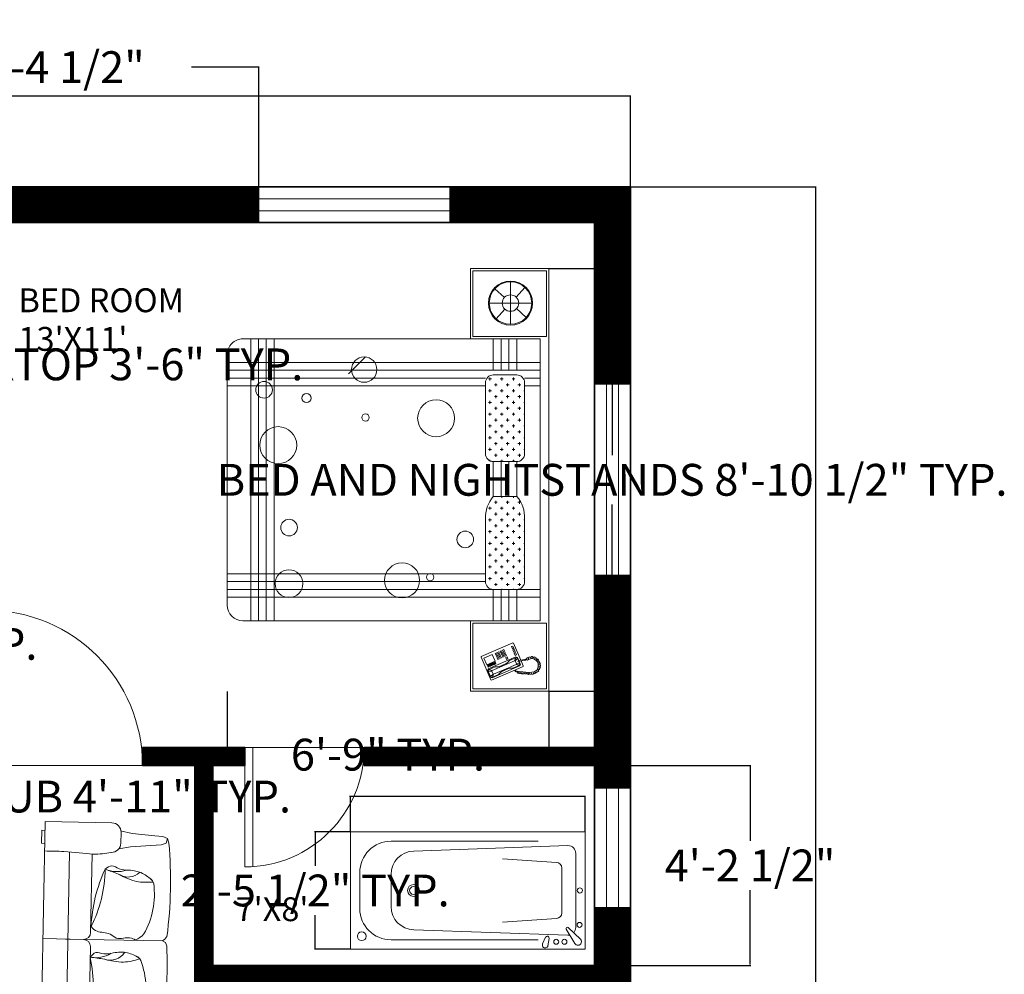
# Model space of a CAD drawing. Units: inches. Extents: x 108 to 771, y 58 to 590.
# Tile 8 of 8: x 524 to 771, y 350 to 590. Entities that reach past the tile are written whole.
import ezdxf

# ---------------------------------------------------------------- set-up
doc = ezdxf.new("R2010")
doc.units = ezdxf.units.IN
doc.header["$MEASUREMENT"] = 0
for name, color, linetype, lineweight in [('A-ANNO-DIMS', 2, 'Continuous', 13), ('A-AREA-IDEN', 7, 'Continuous', 18), ('A-DOOR', 3, 'Continuous', 18), ('A-FLOR-FIXT', 8, 'Continuous', 15), ('A-GLAZ', 4, 'Continuous', 18), ('A-WALL', 7, 'Continuous', 35), ('A-WALL-PATT', 252, 'Continuous', 9), ('Furniture', 7, 'Continuous', 15)]:
    doc.layers.add(name, color=color, linetype=linetype, lineweight=lineweight)
doc.styles.get("Standard").update_dxf_attribs({"font": 'italic8.shx'})
doc.dimstyles.get("Standard").update_dxf_attribs({"dimtxt": 8, "dimasz": 0.18, "dimexe": 0.18, "dimexo": 0.0625, "dimgap": 0.09, "dimtad": 0, "dimtih": 1, "dimtoh": 1, "dimzin": 0, "dimdsep": 46, "dimlunit": 3, "dimtxsty": 'Standard', "dimcen": 0.09, "dimclrt": 6, "dimadec": 0, "dimazin": 0, "dimtfac": 1, "dimtofl": 0, "dimtmove": 0, "dimatfit": 3, "dimfxl": 1, "dimtolj": 1, "dimtzin": 0, "dimarcsym": 0})

# ---------------------------------------------------------------- blocks, each defined once
blk = doc.blocks.new('*D5')
at = {"layer": 'A-ANNO-DIMS', "color": 0, "lineweight": -2, "transparency": 16777216}
for p, q in [((162.35, 548.12), (162.35, 571.05)), ((162.53, 570.87), (386.42, 570.87)), ((677.17, 570.87), (453.27, 570.87)), ((677.35, 548.12), (677.35, 571.05))]:
    blk.add_line(p, q, dxfattribs=at)
at = {"layer": 'A-ANNO-DIMS', "color": 0, "transparency": 16777216}
for points in [[(162.53, 570.9), (162.53, 570.84), (162.35, 570.87)], [(677.17, 570.9), (677.17, 570.84), (677.35, 570.87)]]:
    blk.add_solid(points, dxfattribs=at)
at = {"layer": 'Defpoints', "color": 0, "transparency": 16777216}
for p in [(677.35, 570.87), (162.35, 548.05), (677.35, 548.05)]:
    blk.add_point(p, dxfattribs=at)
at = {"layer": 'A-ANNO-DIMS', "color": 0, "transparency": 16777216, "insert": (419.85, 570.87), "char_height": 8, "attachment_point": 5}
blk.add_mtext('\\A1;42\'-11.00"', dxfattribs=at)
blk = doc.blocks.new('*D6')
at = {"layer": 'A-ANNO-DIMS', "color": 0, "lineweight": -2, "transparency": 16777216}
for p, q in [((677.41, 548.05), (724.06, 548.05)), ((723.88, 547.87), (723.88, 328.9)), ((723.88, 100.23), (723.88, 319.2)), ((677.41, 100.05), (724.06, 100.05))]:
    blk.add_line(p, q, dxfattribs=at)
at = {"layer": 'A-ANNO-DIMS', "color": 0, "transparency": 16777216}
for points in [[(723.85, 547.87), (723.91, 547.87), (723.88, 548.05)], [(723.85, 100.23), (723.91, 100.23), (723.88, 100.05)]]:
    blk.add_solid(points, dxfattribs=at)
at = {"layer": 'Defpoints', "color": 0, "transparency": 16777216}
for p in [(677.35, 548.05), (677.35, 100.05), (723.88, 100.05)]:
    blk.add_point(p, dxfattribs=at)
at = {"layer": 'A-ANNO-DIMS', "color": 0, "transparency": 16777216, "insert": (723.88, 324.05), "char_height": 8, "attachment_point": 5}
blk.add_mtext('\\A1;37\'-4.00"', dxfattribs=at)
blk = doc.blocks.new('DOOR-SINGLE-39')
for p, q in [((0, 39), (0, 0)), ((2, 38.95), (2, 0)), ((0, 0), (39, 0))]:
    blk.add_line(p, q)
blk.add_arc((0, 0), 39, 0, 90)
blk = doc.blocks.new('DOOR-SINGLE-30')
for p, q in [((28, 29.93), (28, 0)), ((30, 30), (30, 0)), ((30, 0), (0, 0))]:
    blk.add_line(p, q)
blk.add_arc((30, 0), 30, 90, 180)
blk = doc.blocks.new('WINDOW-48')
for p, q in [((0, 48), (0, 0)), ((9, 48), (0, 48)), ((3, 48), (3, 0)), ((6, 48), (6, 0)), ((9, 0), (9, 48)), ((0, 0), (9, 0))]:
    blk.add_line(p, q)
blk = doc.blocks.new('WINDOW-30')
for p, q in [((0, 0), (0, 30)), ((0, 30), (9, 30)), ((3, 30), (3, 0)), ((6, 30), (6, 0)), ((9, 30), (9, 0)), ((9, 0), (0, 0))]:
    blk.add_line(p, q)
blk = doc.blocks.new('BED-WITH-NIGHTSTANDS')
h = blk.add_hatch()
h.set_pattern_fill('CROSS', color=256, scale=5.9055, angle=450, style=0)
h.set_pattern_definition([(90, (-724.7189, -618.2251), (1.476375, 1.476375), [0.7381875, -2.2145625]), (360, (-725.088, -617.856), (1.476375, -1.476375), [0.7381875, -2.2145625])])
h.paths.add_polyline_path([(13.93, 48.57), (8.02, 48.57, 0.414214), (6.06, 46.6), (6.06, 28.74, 0.414214), (8.02, 26.77), (13.93, 26.77, 0.414214), (15.9, 28.74), (15.9, 46.6, 0.414214)])
h.paths.add_polyline_path([(6.06, 62.99, 0.19223), (8.02, 57.33), (13.93, 57.33, 0.19223), (15.9, 62.99), (15.9, 78.74, 0.414214), (13.93, 80.71), (8.02, 80.71, 0.414214), (6.06, 78.74)])
for p, q in [((0, 0), (0, 106.3)), ((19.69, 106.3), (0, 106.3)), ((19.09, 105.71), (0.59, 105.71)), ((0.59, 105.71), (0.59, 89.17)), ((19.09, 105.71), (19.09, 89.17)), ((19.69, 106.3), (19.69, 88.58)), ((2.89, 101.55), (3.11, 101.7)), ((3.06, 101.2), (2.89, 101.55)), ((3.11, 101.7), (3.41, 101.48)), ((3.36, 101.88), (3.67, 101.95)), ((3.41, 101.48), (3.36, 101.88)), ((3.67, 101.95), (3.81, 101.64)), ((4.95, 101.56), (3.69, 101.46)), ((3.81, 101.64), (3.94, 101.98)), ((3.94, 101.98), (4.24, 102.02)), ((4.24, 102.02), (4.39, 101.64)), ((4.37, 102.03), (4.76, 102.08)), ((4.39, 101.64), (4.37, 102.03)), ((4.76, 102.08), (4.88, 101.72)), ((4.88, 101.72), (5.13, 102.07)), ((5.79, 101.48), (4.95, 101.56)), ((5.13, 102.07), (5.37, 102.03)), ((5.37, 102.03), (5.42, 101.66)), ((5.42, 101.66), (5.65, 101.97)), ((5.65, 101.97), (5.95, 101.95)), ((5.86, 101.55), (5.79, 101.48)), ((5.92, 101.48), (5.86, 101.55)), ((5.95, 101.95), (5.98, 101.59)), ((5.98, 101.59), (6.16, 101.92)), ((6.16, 101.92), (6.47, 101.91)), ((14.35, 103.55), (6.45, 100.09)), ((6.47, 101.91), (6.46, 101.54)), ((6.46, 101.54), (6.62, 101.9)), ((6.62, 101.9), (6.85, 101.89)), ((6.85, 101.89), (6.89, 101.51)), ((6.89, 101.51), (7.15, 101.84)), ((7.15, 101.84), (7.36, 101.82)), ((14.21, 102.94), (7.34, 99.94)), ((7.36, 101.82), (7.4, 101.48)), ((7.4, 101.48), (7.62, 101.8)), ((7.62, 101.8), (7.77, 101.81)), ((7.77, 101.81), (7.86, 101.7)), ((7.86, 101.7), (7.96, 101.49)), ((11.28, 100.91), (13.85, 102.03)), ((12.15, 101.56), (11.77, 101.33)), ((12.36, 101.86), (12.15, 101.56)), ((12.6, 102.1), (12.36, 101.86)), ((14.14, 102.78), (12.6, 102.1)), ((14.14, 102.78), (13.85, 102.03)), ((13.85, 102.03), (13.99, 102.03)), ((13.99, 102.03), (14.61, 102.64)), ((13.99, 102.03), (14.34, 101.23)), ((14.4, 102.82), (14.14, 102.78)), ((14.62, 102.78), (14.21, 102.94)), ((14.52, 103.48), (14.35, 103.55)), ((14.61, 102.64), (14.4, 102.82)), ((17.02, 97.76), (14.52, 103.48)), ((15.21, 101.26), (14.61, 102.64)), ((15.37, 101.06), (14.62, 102.78)), ((2.06, 100.15), (2.14, 100.41)), ((2.46, 100.04), (2.06, 100.15)), ((2.09, 99.7), (2.1, 99.92)), ((2.44, 99.53), (2.09, 99.7)), ((2.1, 99.92), (2.46, 100.04)), ((2.13, 99.38), (2.44, 99.53)), ((2.17, 99.14), (2.13, 99.38)), ((2.14, 100.41), (2.51, 100.41)), ((2.59, 99.17), (2.17, 99.14)), ((2.23, 100.67), (2.3, 100.88)), ((2.51, 100.41), (2.23, 100.67)), ((2.29, 98.95), (2.59, 99.17)), ((2.3, 100.88), (2.69, 100.86)), ((2.44, 101.15), (2.63, 101.34)), ((2.69, 100.86), (2.44, 101.15)), ((2.89, 100.92), (2.62, 100.19)), ((2.62, 100.19), (2.62, 99.39)), ((2.62, 99.39), (2.98, 98.72)), ((2.63, 101.34), (3.06, 101.2)), ((3.69, 101.46), (2.89, 100.92)), ((6.5, 101.45), (5.92, 101.48)), ((6.45, 100.09), (6.38, 99.93)), ((6.38, 99.93), (6.92, 98.7)), ((7.29, 101.35), (6.5, 101.45)), ((7.34, 99.94), (7.12, 99.5)), ((7.12, 99.5), (7.41, 98.83)), ((7.23, 99.41), (7.24, 99.69)), ((8.09, 99.45), (7.23, 99.41)), ((7.47, 98.85), (7.23, 99.41)), ((7.24, 99.69), (7.44, 99.85)), ((7.73, 101.29), (7.29, 101.35)), ((7.44, 99.85), (8.99, 100.52)), ((7.44, 99.85), (8.18, 99.56)), ((7.79, 101.48), (7.73, 101.29)), ((7.84, 101.37), (7.79, 101.48)), ((7.94, 101.33), (7.84, 101.37)), ((8.11, 101.22), (7.94, 101.33)), ((7.96, 101.49), (8.25, 101.43)), ((8.18, 99.56), (8.09, 99.45)), ((8.09, 99.45), (8.45, 98.65)), ((8.26, 101.14), (8.11, 101.22)), ((11.28, 100.91), (8.18, 99.56)), ((8.25, 101.43), (8.4, 101.32)), ((8.4, 100.95), (8.26, 101.14)), ((8.26, 97.68), (15.18, 100.71)), ((8.4, 101.32), (8.57, 101.02)), ((11.68, 99.99), (8.58, 98.64)), ((8.99, 100.52), (9.33, 100.53)), ((9.33, 100.53), (9.69, 100.49)), ((9.69, 100.49), (10.11, 100.6)), ((10.08, 98.82), (10.29, 99.11)), ((10.11, 100.6), (11.2, 101.08)), ((10.29, 99.11), (10.66, 99.34)), ((10.66, 99.34), (11.75, 99.82)), ((11.77, 101.33), (11.2, 101.08)), ((11.68, 99.99), (14.25, 101.12)), ((12.33, 100.07), (11.75, 99.82)), ((12.75, 100.19), (12.33, 100.07)), ((13.11, 100.14), (12.75, 100.19)), ((13.45, 100.15), (13.11, 100.14)), ((13.3, 99.4), (13.47, 99.48)), ((13.5, 98.95), (13.3, 99.4)), ((15, 100.83), (13.45, 100.15)), ((15.58, 99.65), (13.46, 98.72)), ((13.47, 99.48), (13.67, 99.02)), ((13.64, 99.55), (13.81, 99.63)), ((13.84, 99.1), (13.64, 99.55)), ((13.81, 99.63), (14.01, 99.17)), ((14.01, 99.17), (13.84, 99.1)), ((13.99, 99.7), (14.16, 99.78)), ((14.19, 99.25), (13.99, 99.7)), ((14.16, 99.78), (14.36, 99.32)), ((14.36, 99.32), (14.19, 99.25)), ((14.25, 101.12), (14.34, 101.23)), ((15, 100.83), (14.25, 101.12)), ((14.33, 99.85), (14.5, 99.93)), ((14.53, 99.4), (14.33, 99.85)), ((14.34, 101.23), (15.21, 101.26)), ((14.5, 99.93), (14.7, 99.47)), ((14.7, 99.47), (14.53, 99.4)), ((14.67, 100), (14.84, 100.08)), ((14.87, 99.55), (14.67, 100)), ((14.84, 100.08), (15.04, 99.62)), ((15.04, 99.62), (14.87, 99.55)), ((15.2, 100.99), (15, 100.83)), ((15.02, 100.16), (15.19, 100.23)), ((15.22, 99.7), (15.02, 100.16)), ((15.18, 100.71), (15.37, 101.06)), ((15.19, 100.23), (15.39, 99.77)), ((15.21, 101.26), (15.2, 100.99)), ((15.39, 99.77), (15.22, 99.7)), ((16.3, 97.99), (15.58, 99.65)), ((2.4, 98.76), (2.29, 98.95)), ((2.78, 98.76), (2.4, 98.76)), ((2.53, 98.47), (2.78, 98.76)), ((2.71, 98.26), (2.53, 98.47)), ((3.07, 98.46), (2.71, 98.26)), ((2.96, 98.08), (3.07, 98.46)), ((3.2, 97.92), (2.96, 98.08)), ((2.98, 98.72), (3.58, 98.25)), ((3.49, 98.1), (3.2, 97.92)), ((3.41, 97.75), (3.49, 98.1)), ((3.69, 97.67), (3.41, 97.75)), ((3.58, 98.25), (4.33, 98.05)), ((3.95, 97.97), (3.69, 97.67)), ((4.03, 97.59), (3.95, 97.97)), ((4.36, 97.56), (4.03, 97.59)), ((4.33, 98.05), (5.08, 98.31)), ((4.48, 97.99), (4.36, 97.56)), ((4.67, 97.64), (4.48, 97.99)), ((5, 97.75), (4.67, 97.64)), ((5.05, 98.16), (5, 97.75)), ((5.26, 97.85), (5.05, 98.16)), ((5.08, 98.31), (5.33, 98.48)), ((5.53, 98), (5.26, 97.85)), ((5.33, 98.48), (5.57, 98.34)), ((5.6, 98.18), (5.53, 98)), ((5.57, 98.34), (5.87, 98.48)), ((5.68, 98.18), (5.6, 98.18)), ((5.98, 98.32), (5.68, 98.18)), ((5.87, 98.48), (6.16, 98.57)), ((6.58, 98.42), (5.98, 98.32)), ((6.16, 98.57), (6.77, 98.66)), ((7.22, 98.53), (6.58, 98.42)), ((6.77, 98.66), (7.17, 98.75)), ((7.01, 98.5), (8.89, 94.2)), ((7.17, 98.75), (7.65, 98.91)), ((7.72, 98.74), (7.22, 98.53)), ((7.49, 98.64), (7.84, 97.84)), ((7.83, 98.04), (7.55, 98.67)), ((7.65, 98.91), (7.72, 98.74)), ((8.45, 98.65), (7.83, 98.04)), ((7.83, 98.04), (8.04, 97.86)), ((7.84, 97.84), (8.26, 97.68)), ((8.04, 97.86), (8.29, 97.9)), ((8.09, 97.13), (8.43, 97.28)), ((8.34, 96.55), (8.09, 97.13)), ((8.29, 97.9), (8.58, 98.64)), ((8.29, 97.9), (9.84, 98.58)), ((8.68, 96.7), (8.34, 96.55)), ((8.43, 97.28), (8.68, 96.7)), ((8.58, 98.64), (8.45, 98.65)), ((9.05, 94.14), (16.96, 97.59)), ((9.84, 98.58), (10.08, 98.82)), ((10.58, 98.29), (10.24, 98.14)), ((10.24, 98.14), (10.44, 97.68)), ((10.44, 97.68), (10.78, 97.83)), ((10.78, 97.83), (10.58, 98.29)), ((10.93, 97.48), (10.59, 97.33)), ((10.59, 97.33), (10.74, 96.99)), ((10.74, 96.99), (11.08, 97.14)), ((11.18, 96.91), (10.84, 96.76)), ((10.84, 96.76), (10.99, 96.42)), ((11.08, 97.14), (10.93, 97.48)), ((11.33, 96.57), (11.18, 96.91)), ((11.56, 97.76), (11.22, 97.61)), ((11.22, 97.61), (11.37, 97.27)), ((11.37, 97.27), (11.71, 97.42)), ((11.81, 97.19), (11.47, 97.04)), ((11.47, 97.04), (11.62, 96.69)), ((11.71, 97.42), (11.56, 97.76)), ((11.62, 96.69), (11.96, 96.84)), ((12.06, 96.61), (11.72, 96.46)), ((11.96, 96.84), (11.81, 97.19)), ((12.19, 98.03), (11.85, 97.88)), ((11.85, 97.88), (12, 97.54)), ((12, 97.54), (12.34, 97.69)), ((12.21, 96.27), (12.06, 96.61)), ((12.44, 97.46), (12.1, 97.31)), ((12.1, 97.31), (12.25, 96.97)), ((12.34, 97.69), (12.19, 98.03)), ((12.25, 96.97), (12.59, 97.12)), ((12.69, 96.89), (12.35, 96.74)), ((12.35, 96.74), (12.5, 96.39)), ((12.59, 97.12), (12.44, 97.46)), ((12.82, 98.31), (12.48, 98.16)), ((12.48, 98.16), (12.63, 97.82)), ((12.63, 97.82), (12.97, 97.97)), ((12.84, 96.55), (12.69, 96.89)), ((13.07, 97.74), (12.73, 97.59)), ((12.73, 97.59), (12.88, 97.24)), ((12.97, 97.97), (12.82, 98.31)), ((12.88, 97.24), (13.22, 97.39)), ((13.32, 97.16), (12.98, 97.01)), ((12.98, 97.01), (13.13, 96.67)), ((13.22, 97.39), (13.07, 97.74)), ((13.13, 96.67), (13.47, 96.82)), ((13.47, 96.82), (13.32, 97.16)), ((13.46, 98.72), (14.18, 97.06)), ((13.67, 99.02), (13.5, 98.95)), ((14.18, 97.06), (16.3, 97.99)), ((16.96, 97.59), (17.02, 97.76)), ((8.44, 96.33), (8.78, 96.48)), ((8.69, 95.75), (8.44, 96.33)), ((9.03, 95.9), (8.69, 95.75)), ((8.78, 96.48), (9.03, 95.9)), ((8.79, 95.52), (9.13, 95.67)), ((9.04, 94.95), (8.79, 95.52)), ((8.89, 94.2), (9.05, 94.14)), ((9.38, 95.1), (9.04, 94.95)), ((9.13, 95.67), (9.38, 95.1)), ((10.99, 96.42), (11.33, 96.57)), ((11.43, 96.34), (11.09, 96.19)), ((11.09, 96.19), (11.24, 95.84)), ((11.24, 95.84), (11.58, 95.99)), ((11.58, 95.99), (11.43, 96.34)), ((11.72, 96.46), (11.87, 96.12)), ((11.87, 96.12), (12.21, 96.27)), ((12.5, 96.39), (12.84, 96.55)), ((19.09, 89.17), (0.59, 89.17)), ((0.59, 89.17), (19.09, 89.17)), ((2.12, 17.72), (2.12, 88.58)), ((2.12, 88.58), (76.92, 88.58)), ((80.86, 84.65), (80.86, 21.65)), ((55.34, 82.68), (55.28, 82.62)), ((6.07, 78.98), (6.07, 62.76)), ((6.07, 46.84), (6.07, 28.51)), ((6.07, 44.57), (6.06, 44.56)), ((50.36, 26.51), (46.1, 22.26)), ((76.92, 17.72), (2.12, 17.72)), ((19.69, 0), (19.69, 17.72)), ((19.09, 17.13), (0.59, 17.13)), ((0.59, 0.59), (0.59, 17.13)), ((19.09, 0.59), (19.09, 17.13)), ((9.61, 8.71), (9.61, 14.05)), ((11, 10.24), (13.2, 12.67)), ((8.07, 10.1), (5.65, 12.3)), ((9.61, 8.71), (4.26, 8.71)), ((9.61, 8.71), (14.95, 8.71)), ((9.61, 8.71), (9.61, 3.36)), ((8.22, 7.18), (6.02, 4.75)), ((11.14, 7.32), (13.56, 5.12)), ((19.69, 0), (0, 0)), ((19.09, 0.59), (0.59, 0.59))]:
    blk.add_line(p, q)
for points in [[(8.02, 88.58), (8.02, 80.71)], [(9.99, 80.71), (9.99, 88.58), (8.02, 88.58)], [(13.93, 80.71), (13.93, 88.58), (11.96, 88.58)], [(11.96, 88.58), (11.96, 80.71)], [(2.12, 80.71), (80.86, 80.71), (80.86, 82.68), (2.12, 82.68)], [(15.9, 76.77), (80.86, 76.77), (80.86, 78.74), (15.9, 78.74)], [(8.02, 57.33), (8.02, 48.57)], [(9.99, 48.57), (9.99, 57.33)], [(11.96, 57.33), (11.96, 48.57)], [(13.93, 48.57), (13.93, 57.33)], [(2.12, 29.53), (6.06, 29.53)], [(6.06, 27.56), (2.12, 27.56)], [(15.9, 29.53), (80.86, 29.53), (80.86, 27.56), (15.9, 27.56)], [(2.12, 25.59), (80.86, 25.59), (80.86, 23.62), (2.12, 23.62)], [(8.02, 25.59), (8.02, 17.72), (9.99, 17.72), (9.99, 25.59)], [(11.96, 25.59), (11.96, 17.72), (13.93, 17.72), (13.93, 25.59)]]:
    blk.add_lwpolyline(points)
for points in [[(69.05, 88.58), (69.05, 17.72), (71.02, 17.72), (71.02, 88.58)], [(72.98, 88.58), (72.98, 17.72), (74.95, 17.72), (74.95, 88.58)]]:
    blk.add_lwpolyline(points, close=True)
for points in [[(15.9, 62.99), (15.9, 78.74, 0.414214), (13.93, 80.71), (8.02, 80.71, 0.414214), (6.06, 78.74), (6.06, 62.99, 0.19223), (8.02, 57.33), (13.93, 57.33, 0.19223)], [(15.9, 28.74), (15.9, 46.6, 0.414214), (13.93, 48.57), (8.02, 48.57, 0.414214), (6.06, 46.6), (6.06, 28.74, 0.414214), (8.02, 26.77), (13.93, 26.77, 0.414214)]]:
    blk.add_lwpolyline(points, format="xyb", close=True)
for centre, radius in [((36.86, 78.44), 4.41), ((65.32, 79.25), 3.48), ((29.81, 77.62), 0.925), ((20.97, 68.13), 2.09), ((65.3, 65.16), 2.09), ((68.02, 44.43), 4.65), ((28.31, 37.66), 4.65), ((46.05, 37.48), 0.925), ((60.91, 32.6), 1.14), ((71.58, 30.51), 2.09), ((46.4, 25.43), 3.19), ((9.61, 8.71), 5.54), ((9.61, 8.71), 5.34), ((9.61, 8.71), 2.07)]:
    blk.add_circle(centre, radius)
for centre, start, end in [((76.92, 84.65), 0, 90), ((76.92, 21.65), 270, 0)]:
    blk.add_arc(centre, 3.94, start, end)
blk = doc.blocks.new('BATHTUB')
for p, q in [((59.06, 29.53), (0, 29.53)), ((0, 29.53), (0, 0)), ((4.78, 24.45), (2.59, 28.08)), ((9.35, 28.65), (9.04, 26.82)), ((9.94, 26.54), (10.7, 28.16)), ((59.06, 0), (59.06, 29.53)), ((1.15, 27.02), (4.3, 24.06)), ((4.33, 26.04), (43.12, 24.68)), ((48.82, 27.17), (11.81, 27.17)), ((2.36, 24.07), (2.36, 5.46)), ((7.23, 21.79), (20.76, 22.69)), ((5.85, 20.41), (5.85, 9.11)), ((48.82, 10.75), (48.82, 19.29)), ((56.69, 10.24), (56.69, 19.29)), ((7.23, 7.74), (20.76, 6.84)), ((4.33, 3.49), (43.12, 4.85)), ((0, 0), (59.06, 0)), ((11.81, 2.36), (48.82, 2.36))]:
    blk.add_line(p, q)
for centre, radius in [((5.23, 27.66), 0.628), ((7.29, 27.66), 0.628), ((56.21, 26.29), 1.09), ((1.42, 23.41), 0.628), ((1.34, 14.76), 0.656), ((43.18, 14.76), 1.48), ((43.18, 14.76), 0.984)]:
    blk.add_circle(centre, radius)
for centre, radius, start, end in [((1.81, 27.63), 0.903, 29.9808, 223.0225), ((10.05, 28.48), 0.722, 333.7022, 166.7439), ((4.33, 24.07), 1.97, 137.6863, 180), ((4.33, 24.07), 1.97, 137.6863, 180), ((4.33, 24.07), 1.97, 90, 103.842), ((4.33, 24.07), 1.97, 90, 103.842), ((9.51, 26.74), 0.472, 170.4963, 334.8002), ((48.82, 19.29), 7.87, 0, 90), ((4.51, 24.29), 0.315, 226.7749, 31.0788), ((4.51, 24.29), 0.315, 226.7749, 31.0788), ((42.91, 18.78), 5.91, 0, 87.9984), ((7.23, 20.41), 1.38, 90, 180), ((42.91, 10.75), 5.91, 272.0016, 0), ((48.82, 10.24), 7.87, 270, 0), ((7.23, 9.11), 1.38, 180, 270), ((4.33, 5.46), 1.97, 180, 270)]:
    blk.add_arc(centre, radius, start, end)
blk = doc.blocks.new('SOFA')
for p, q in [((13.53, 80.95), (2.06, 78.82)), ((12.83, 79.28), (12.82, 76.57)), ((31.83, 81.57, 13.5), (15.2, 81.57, 13.5)), ((31.83, 81.57, 13.5), (31.83, 0)), ((31.83, 79.37, 0.36), (32.62, 79.37, 0.36)), ((32.62, 79.37, 0.36), (32.62, 76.1, 0.36)), ((1.33, 77.65), (1.12, 78.32)), ((2.53, 77.19), (1.33, 77.65)), ((4.58, 77.03), (2.53, 77.19)), ((10.24, 76.55), (4.58, 77.03)), ((12.88, 76.04), (10.24, 76.55)), ((32.62, 76.1, 0.36), (31.83, 76.1, 0.91)), ((19.88, 73.73), (19.88, 54.83)), ((25.57, 7.53, 9.89), (25.57, 74.14, 9.89)), ((1.09, 53.34), (0.67, 54.21)), ((1.09, 52.77), (0.68, 51.91)), ((1.64, 53.06), (1.09, 53.34)), ((1.64, 53.06), (1.09, 52.77)), ((1.64, 53.06), (2.64, 53.06)), ((19.09, 53.06), (21.65, 53.06)), ((21.65, 53.06), (31.83, 53.06)), ((19.88, 51.29), (19.88, 31.21)), ((1.05, 29.87), (0.64, 30.74)), ((1.8, 29.44), (1.05, 29.87)), ((1.19, 29.01), (0.68, 28.32)), ((1.81, 29.44), (1.19, 29.01)), ((26.18, 29.43), (1.8, 29.43)), ((19.88, 27.66), (19.89, 7.88, 0.34)), ((31.83, 29.43), (21.65, 29.43)), ((2.53, 5.3), (1.33, 4.84)), ((10.24, 5.94), (2.53, 5.3)), ((13.2, 6.51), (10.24, 5.94)), ((12.69, 2.37), (12.69, 5.08)), ((32.62, 5.47, 0.36), (31.83, 5.47, 0.91)), ((32.62, 2.2, 0.36), (32.62, 5.47, 0.36)), ((0.97, 3.69), (0.62, 4.84)), ((1.33, 4.84), (0.97, 3.69)), ((2.18, 3.23), (0.97, 3.69)), ((4.22, 3.07), (2.18, 3.23)), ((9.88, 2.59), (4.22, 3.07)), ((12.84, 2.01), (9.88, 2.59)), ((15.05, 0.01), (31.83, 0)), ((31.83, 2.2, 0.36), (32.62, 2.2, 0.36))]:
    blk.add_line(p, q)
for centre, radius, start, end in [((15.09, 79.31, 13.5), 2.25, 87.0581, 180.9206), ((123.26, 65.95), 123.14, 174.6632, 185.4698), ((2.39, 77.08), 1.77, 100.5091, 180), ((-121.91, 65.95), 123.14, 354.5302, 5.3368), ((15.19, 76.56), 2.36, 179.7859, 269.7859), ((19.84, 46.39, 13.5), 19.99, 113.7986, 151.3924), ((12.86, 58.3, 13.5), 6.47, 76.1804, 99.6612), ((3.85, 55.11, 13.5), 1.77, 151.3924, 203.2188), ((36.72, 25.19, 13.5), 33.78, 119.8342, 142.4564), ((21.65, 54.83), 1.77, 180, 270), ((-6.19, 75.47, 13.5), 33.78, 298.4934, 321.1155), ((21.65, 51.29), 1.77, 90, 180), ((315.61, 40.74), 315.13, 177.9678, 181.8181), ((3.98, 47.34, 13.5), 4.27, 21.4614, 98.0497), ((25.7, 41.94, 13.5), 19.99, 164.3829, 201.9767), ((3.65, 42.24, 13.5), 7.21, 29.4203, 72.7126), ((12.07, 44.11, 13.5), 6.47, 142.7695, 150.2454), ((52.79, 41.52, 13.5), 33.78, 166.9593, 193.0407), ((8.8, 35.12, 13.5), 1.77, 201.9767, 253.8031), ((14.9, 30.29, 13.5), 4.27, 72.0456, 148.634), ((18.62, 26.79, 13.5), 7.21, 80.0046, 123.2969), ((21.65, 31.21), 1.77, 180, 270), ((107.05, 16.32), 107.05, 173.5605, 186.1533), ((24, 18.21, 13.5), 19.99, 151.3169, 188.9106), ((11.21, 23.4, 13.5), 6.47, 113.6986, 137.1794), ((21.65, 27.66), 1.77, 90, 180), ((-18.44, 27.22, 13.5), 38.25, 336.0331, 358.4688), ((50.29, 11.67, 13.5), 33.78, 154.5272, 179.9746), ((6, 15.39, 13.5), 1.77, 188.9106, 240.7371), ((10.84, 9.3, 13.5), 4.27, 58.9796, 135.568), ((13.68, 5.05, 13.5), 7.21, 66.9386, 110.2309), ((15.05, 5.08), 2.36, 90, 180), ((15.05, 2.37), 2.36, 180, 269.9816)]:
    blk.add_arc(centre, radius, start, end)
for points, knots in [([(15.18, 74.2), (16.54, 73.96, 2.2), (19.42, 73.44, 6.84), (25.93, 74.31, 10.25), (30.21, 74.29, 11.73), (31.83, 74.28, 12.29)], [0, 0, 0, 0, 7.670782, 16.13452, 21.306634, 21.306634, 21.306634, 21.306634]), ([(14.41, 64.59, 13.5), (14.41, 64.59, 13.5), (15.3, 62.57, 13.5), (18.13, 62.25, 13.5), (18.49, 59.48, 13.5), (19.41, 58.61, 13.5), (19.88, 58.17, 13.5)], [27.786417, 27.786417, 27.786417, 27.786417, 60.334214, 153.42843, 198.910048, 250.027656, 250.027656, 250.027656, 250.027656]), ([(2.08, 55.2, 13.5), (2.3, 54.16, 13.5), (2.79, 51.93, 13.5), (4.99, 49.65, 13.5), (7.18, 48.12, 13.5), (7.83, 45.76, 13.5), (9.25, 45.77, 13.5), (9.93, 45.78, 13.5)], [0, 0, 0, 0, 3.139621, 6.721226, 9.134784, 11.147372, 12.969489, 12.969489, 12.969489, 12.969489]), ([(2.23, 55.48, 13.5), (3.39, 54.7, 13.5), (5.91, 53.01, 13.5), (7.71, 49.11, 13.5), (9.26, 46.77, 13.5), (9.93, 45.78, 13.5)], [0, 0, 0, 0, 4.104513, 8.93575, 12.539242, 12.539242, 12.539242, 12.539242]), ([(15.26, 49.37, 13.5), (16.21, 49.3, 13.5), (17.85, 49.84, 13.5), (19.2, 49.22, 13.5), (19.79, 48.78, 13.5)], [214.332348, 214.332348, 214.332348, 214.332348, 289.238615, 341.466319, 341.466319, 341.466319, 341.466319]), ([(7.49, 34.11, 13.5), (8.83, 34.51, 13.5), (11.73, 35.38, 13.5), (15.9, 34.29, 13.5), (18.69, 34.01, 13.5), (19.88, 33.9, 13.5)], [0, 0, 0, 0, 4.104513, 8.93575, 12.539242, 12.539242, 12.539242, 12.539242]), ([(7.62, 33.81, 13.5), (8.56, 33.33, 13.5), (10.59, 32.29, 13.5), (13.75, 32.54, 13.5), (16.32, 33.26, 13.5), (18.56, 32.26, 13.5), (19.45, 33.37, 13.5), (19.88, 33.9, 13.5)], [0, 0, 0, 0, 3.139621, 6.721226, 9.134784, 11.147372, 12.969489, 12.969489, 12.969489, 12.969489]), ([(8.61, 29.33, 13.5), (8.61, 29.33, 13.5), (10.55, 28.27, 13.5), (12.98, 29.74, 13.5), (15.37, 27.37, 13.5), (18, 27.79, 13.5), (19.32, 26.76, 13.5), (19.79, 26.2, 13.5)], [27.786417, 27.786417, 27.786417, 27.786417, 60.334214, 153.42843, 198.910048, 289.238615, 341.466319, 341.466319, 341.466319, 341.466319]), ([(4.5, 14.7, 13.5), (5.89, 14.78, 13.5), (8.91, 14.98, 13.5), (12.72, 12.97, 13.5), (15.38, 12.07, 13.5), (16.51, 11.69, 13.5)], [0, 0, 0, 0, 4.104513, 8.93575, 12.539242, 12.539242, 12.539242, 12.539242]), ([(4.55, 14.37, 13.5), (5.36, 13.69, 13.5), (7.1, 12.22, 13.5), (10.24, 11.75, 13.5), (12.91, 11.87, 13.5), (14.86, 10.39, 13.5), (15.98, 11.27, 13.5), (16.51, 11.69, 13.5)], [0, 0, 0, 0, 3.139621, 6.721226, 9.134784, 11.147372, 12.969489, 12.969489, 12.969489, 12.969489]), ([(15.18, 7.47), (16.54, 7.71, 2.2), (19.42, 8.23, 6.84), (25.93, 7.36, 10.25), (30.21, 7.38, 11.73), (31.83, 7.39, 12.29)], [0, 0, 0, 0, 7.670782, 16.13452, 21.306634, 21.306634, 21.306634, 21.306634])]:
    blk.add_open_spline(points, degree=3, knots=knots)
blk = doc.blocks.new('*D26')
at = {"layer": 'A-ANNO-DIMS', "color": 0, "lineweight": -2, "transparency": 16777216}
for p, q in [((336.68, 438.49), (336.68, 432.97)), ((372.68, 438.49), (372.68, 432.97)), ((336.86, 433.15), (372.5, 433.15)), ((372.68, 433.15), (372.86, 433.15))]:
    blk.add_line(p, q, dxfattribs=at)
at = {"layer": 'A-ANNO-DIMS', "color": 0, "transparency": 16777216}
for points in [[(336.86, 433.18), (336.86, 433.12), (336.68, 433.15)], [(372.5, 433.18), (372.5, 433.12), (372.68, 433.15)]]:
    blk.add_solid(points, dxfattribs=at)
at = {"layer": 'Defpoints', "color": 0, "transparency": 16777216}
for p in [(336.68, 438.55), (372.68, 438.55), (372.68, 433.15)]:
    blk.add_point(p, dxfattribs=at)
at = {"layer": 'A-ANNO-DIMS', "color": 6, "transparency": 16777216, "insert": (463.04, 433.15), "char_height": 8, "attachment_point": 5}
blk.add_mtext('\\A1;KITCHEN DOOR 3\'-0" TYP.', dxfattribs=at)
blk = doc.blocks.new('*D36')
at = {"layer": 'A-ANNO-DIMS', "color": 0, "lineweight": -2, "transparency": 16777216}
for p, q in [((656.87, 527.54), (672.93, 527.54)), ((672.75, 527.36), (672.75, 480.57)), ((672.75, 421.42), (672.75, 468.2)), ((656.87, 421.24), (672.93, 421.24))]:
    blk.add_line(p, q, dxfattribs=at)
at = {"layer": 'A-ANNO-DIMS', "color": 0, "transparency": 16777216}
for points in [[(672.72, 527.36), (672.78, 527.36), (672.75, 527.54)], [(672.72, 421.42), (672.78, 421.42), (672.75, 421.24)]]:
    blk.add_solid(points, dxfattribs=at)
at = {"layer": 'Defpoints', "color": 0, "transparency": 16777216}
for p in [(656.81, 527.54), (656.81, 421.24), (672.75, 421.24)]:
    blk.add_point(p, dxfattribs=at)
at = {"layer": 'A-ANNO-DIMS', "color": 6, "transparency": 16777216, "insert": (672.75, 474.39), "char_height": 8, "attachment_point": 5}
blk.add_mtext('\\A1;BED AND NIGHTSTANDS 8\'-10 1/2" TYP.', dxfattribs=at)
blk = doc.blocks.new('*D37')
at = {"layer": 'A-ANNO-DIMS', "color": 0, "lineweight": -2, "transparency": 16777216}
for p, q in [((575.95, 421.17), (575.95, 405.11)), ((656.81, 421.17), (656.81, 405.11)), ((576.13, 405.29), (580.1, 405.29)), ((656.63, 405.29), (652.66, 405.29))]:
    blk.add_line(p, q, dxfattribs=at)
at = {"layer": 'A-ANNO-DIMS', "color": 0, "transparency": 16777216}
for points in [[(576.13, 405.32), (576.13, 405.26), (575.95, 405.29)], [(656.63, 405.32), (656.63, 405.26), (656.81, 405.29)]]:
    blk.add_solid(points, dxfattribs=at)
at = {"layer": 'Defpoints', "color": 0, "transparency": 16777216}
for p in [(575.95, 421.24), (656.81, 421.24), (575.95, 405.29)]:
    blk.add_point(p, dxfattribs=at)
at = {"layer": 'A-ANNO-DIMS', "color": 6, "transparency": 16777216, "insert": (616.38, 405.29), "char_height": 8, "attachment_point": 5}
blk.add_mtext('\\A1;6\'-9" TYP.', dxfattribs=at)
blk = doc.blocks.new('*D38')
at = {"layer": 'A-ANNO-DIMS', "color": 0, "lineweight": -2, "transparency": 16777216}
for p, q in [((606.93, 394.75), (606.75, 394.75)), ((606.93, 385.95), (606.93, 394.93)), ((665.8, 394.75), (607.11, 394.75)), ((665.98, 385.95), (665.98, 394.93))]:
    blk.add_line(p, q, dxfattribs=at)
at = {"layer": 'A-ANNO-DIMS', "color": 0, "transparency": 16777216}
for points in [[(607.11, 394.78), (607.11, 394.72), (606.93, 394.75)], [(665.8, 394.78), (665.8, 394.72), (665.98, 394.75)]]:
    blk.add_solid(points, dxfattribs=at)
at = {"layer": 'Defpoints', "color": 0, "transparency": 16777216}
for p in [(606.93, 394.75), (606.93, 385.89), (665.98, 385.89)]:
    blk.add_point(p, dxfattribs=at)
at = {"layer": 'A-ANNO-DIMS', "color": 6, "transparency": 16777216, "insert": (552.56, 394.75), "char_height": 8, "attachment_point": 5}
blk.add_mtext('\\A1;TUB 4\'-11" TYP.', dxfattribs=at)
blk = doc.blocks.new('*D39')
at = {"layer": 'A-ANNO-DIMS', "color": 0, "lineweight": -2, "transparency": 16777216}
for p, q in [((606.86, 385.89), (597.89, 385.89)), ((598.07, 385.71), (598.07, 377.31)), ((598.07, 356.54), (598.07, 364.94)), ((606.86, 356.36), (597.89, 356.36))]:
    blk.add_line(p, q, dxfattribs=at)
at = {"layer": 'A-ANNO-DIMS', "color": 0, "transparency": 16777216}
for points in [[(598.04, 385.71), (598.1, 385.71), (598.07, 385.89)], [(598.04, 356.54), (598.1, 356.54), (598.07, 356.36)]]:
    blk.add_solid(points, dxfattribs=at)
at = {"layer": 'Defpoints', "color": 0, "transparency": 16777216}
for p in [(606.93, 385.89), (598.07, 356.36), (606.93, 356.36)]:
    blk.add_point(p, dxfattribs=at)
at = {"layer": 'A-ANNO-DIMS', "color": 6, "transparency": 16777216, "insert": (598.07, 371.13), "char_height": 8, "attachment_point": 5}
blk.add_mtext('\\A1;2\'-5 1/2" TYP.', dxfattribs=at)
blk = doc.blocks.new('*D40')
at = {"layer": 'A-ANNO-DIMS', "color": 0, "lineweight": -2, "transparency": 16777216}
for p, q in [((432.85, 509.64), (432.85, 503.24)), ((474.74, 509.64), (474.74, 503.24)), ((433.03, 503.42), (474.56, 503.42)), ((474.74, 503.42), (474.92, 503.42))]:
    blk.add_line(p, q, dxfattribs=at)
at = {"layer": 'A-ANNO-DIMS', "color": 0, "transparency": 16777216}
for points in [[(433.03, 503.45), (433.03, 503.39), (432.85, 503.42)], [(474.56, 503.45), (474.56, 503.39), (474.74, 503.42)]]:
    blk.add_solid(points, dxfattribs=at)
at = {"layer": 'Defpoints', "color": 0, "transparency": 16777216}
for p in [(432.85, 509.7), (474.74, 509.7), (474.74, 503.42)]:
    blk.add_point(p, dxfattribs=at)
at = {"layer": 'A-ANNO-DIMS', "color": 6, "transparency": 16777216, "insert": (543.58, 503.42), "char_height": 8, "attachment_point": 5}
blk.add_mtext('\\A1;COOKTOP 3\'-6" TYP.', dxfattribs=at)
blk = doc.blocks.new('*D51')
at = {"layer": 'A-ANNO-DIMS', "color": 0, "lineweight": -2, "transparency": 16777216}
for p, q in [((668.41, 402.55), (707.63, 402.55)), ((707.45, 402.37), (707.45, 383.61)), ((707.45, 352.48), (707.45, 371.24)), ((668.41, 352.3), (707.63, 352.3))]:
    blk.add_line(p, q, dxfattribs=at)
at = {"layer": 'A-ANNO-DIMS', "color": 0, "transparency": 16777216}
for points in [[(707.42, 402.37), (707.48, 402.37), (707.45, 402.55)], [(707.42, 352.48), (707.48, 352.48), (707.45, 352.3)]]:
    blk.add_solid(points, dxfattribs=at)
at = {"layer": 'Defpoints', "color": 0, "transparency": 16777216}
for p in [(668.35, 402.55), (707.45, 402.55), (668.35, 352.3)]:
    blk.add_point(p, dxfattribs=at)
at = {"layer": 'A-ANNO-DIMS', "color": 6, "transparency": 16777216, "insert": (707.45, 377.43), "char_height": 8, "attachment_point": 5}
blk.add_mtext('\\A1;4\'-2 1/2"', dxfattribs=at)
blk = doc.blocks.new('*D56')
at = {"layer": 'A-ANNO-DIMS', "color": 0, "lineweight": -2, "transparency": 16777216}
for p, q in [((483.58, 548.12), (483.58, 578.33)), ((483.76, 578.15), (500.52, 578.15)), ((583.74, 578.15), (566.98, 578.15)), ((583.92, 548.12), (583.92, 578.33))]:
    blk.add_line(p, q, dxfattribs=at)
at = {"layer": 'A-ANNO-DIMS', "color": 0, "transparency": 16777216}
for points in [[(483.76, 578.18), (483.76, 578.12), (483.58, 578.15)], [(583.74, 578.18), (583.74, 578.12), (583.92, 578.15)]]:
    blk.add_solid(points, dxfattribs=at)
at = {"layer": 'Defpoints', "color": 0, "transparency": 16777216}
for p in [(583.92, 578.15), (483.58, 548.05), (583.92, 548.05)]:
    blk.add_point(p, dxfattribs=at)
at = {"layer": 'A-ANNO-DIMS', "color": 6, "transparency": 16777216, "insert": (533.75, 578.15), "char_height": 8, "attachment_point": 5}
blk.add_mtext('\\A1;8\'-4 1/2"', dxfattribs=at)

msp = doc.modelspace()

# ---------------------------------------------------------------- hatches: boundary and pattern name
at = {"layer": 'A-WALL-PATT'}
h = msp.add_hatch(dxfattribs=at)
h.set_pattern_fill('ANSI31', color=256)
h.paths.add_polyline_path([(171.345, 461.548), (162.345, 461.548), (162.345, 390.901), (171.345, 390.901), (171.345, 393.51), (171.345, 402.553), (233.142, 402.553), (233.142, 407.053), (171.345, 407.053)])
h.paths.add_polyline_path([(331.845, 438.553), (336.68, 438.554), (336.68, 443.053), (331.845, 443.053), (331.845, 539.053), (365.02, 539.053), (365.02, 548.053), (280.772, 548.053), (280.772, 539.053), (327.345, 539.053), (327.345, 407.053), (325.63, 407.053), (325.63, 402.553), (331.845, 402.553)])
h.paths.add_polyline_path([(286.63, 407.053), (263.142, 407.053), (263.142, 402.553), (267.345, 402.553), (267.345, 352.303), (171.345, 352.303), (171.345, 360.901), (162.345, 360.901), (162.345, 336.026), (171.345, 336.026), (171.345, 347.803), (267.345, 347.803), (267.345, 293.053), (263.142, 293.053), (263.142, 288.553), (293.037, 288.553), (293.037, 293.053), (271.845, 293.053), (271.845, 402.553), (286.63, 402.553)])
h.paths.add_polyline_path([(466.018, 443.053), (424.345, 443.053), (424.345, 539.053), (453.584, 539.053), (453.584, 548.053), (395.02, 548.053), (395.02, 539.053), (419.845, 539.053), (420.71, 443.053), (372.68, 443.053), (372.68, 438.557), (420.751, 438.561), (421.075, 402.553), (422.061, 293.053), (419.994, 293.053), (419.994, 288.553), (426.124, 288.553), (426.124, 293.053), (424.345, 293.053), (424.345, 402.553), (424.345, 438.553), (466.018, 438.553)])
h.paths.add_polyline_path([(512.345, 539.053), (583.918, 539.053), (583.918, 548.053), (483.584, 548.053), (483.584, 539.053), (507.845, 539.053), (507.845, 443.053), (502.018, 443.053), (502.018, 438.553), (507.845, 438.553), (507.845, 402.553), (515.658, 402.553), (515.658, 407.053), (512.345, 407.053)])
h.paths.add_polyline_path([(232.772, 548.053), (162.345, 548.053), (162.345, 509.548), (171.345, 509.548), (171.345, 539.053), (232.772, 539.053)])
h.paths.add_polyline_path([(233.142, 293.053), (171.345, 293.053), (171.345, 306.026), (162.345, 306.026), (162.345, 230.8), (171.345, 230.8), (171.345, 288.553), (233.142, 288.553)])
h.paths.add_polyline_path([(359.994, 293.053), (332.037, 293.053), (332.037, 288.553), (339.345, 288.553), (339.345, 145.053), (334.469, 145.053), (334.469, 136.053), (339.345, 136.053), (339.345, 104.553), (166.845, 104.553), (166.845, 136.053), (211.837, 136.053), (211.837, 145.053), (171.345, 145.053), (171.345, 182.8), (162.345, 182.8), (162.345, 100.053), (343.845, 100.053), (343.845, 136.053), (400.886, 136.053), (400.886, 145.053), (348.345, 145.053), (348.345, 288.553), (359.994, 288.553)])
h.paths.add_polyline_path([(500.345, 288.553), (503.755, 288.553), (503.755, 293.053), (486.124, 293.053), (486.124, 288.553), (491.345, 288.553), (491.345, 145.053), (448.886, 145.053), (448.886, 136.053), (495.845, 136.053), (495.845, 100.053), (677.345, 100.053), (677.345, 186.265), (668.345, 186.265), (668.345, 145.053), (627.637, 145.053), (627.637, 136.053), (672.845, 136.053), (672.845, 104.278), (500.345, 104.539), (500.345, 136.053), (504.239, 136.053), (504.239, 145.053), (500.345, 145.053)])
h.paths.add_polyline_path([(580.913, 293.053), (572.345, 293.053), (572.345, 347.803), (668.345, 347.803), (668.345, 330.831), (677.345, 330.831), (677.345, 366.853), (668.345, 366.853), (668.345, 352.303), (572.345, 352.303), (572.345, 402.553), (580.418, 402.553), (580.418, 407.053), (554.658, 407.053), (554.658, 402.553), (567.845, 402.553), (567.845, 293.053), (542.755, 293.053), (542.755, 288.553), (580.913, 288.553)])
h.paths.add_polyline_path([(677.345, 300.831), (668.345, 300.831), (668.345, 293.053), (610.913, 293.053), (610.913, 288.553), (668.345, 288.553), (668.345, 234.265), (677.345, 234.265)])
h.paths.add_polyline_path([(304.469, 145.053), (259.837, 145.053), (259.837, 136.053), (304.469, 136.053)], flags=17)
h.paths.add_polyline_path([(579.637, 145.053), (534.239, 145.053), (534.239, 136.053), (579.637, 136.053)], flags=17)
h.paths.add_polyline_path([(677.345, 450.416), (668.345, 450.416), (668.345, 407.053), (610.418, 407.053), (610.418, 402.553), (668.345, 402.553), (668.345, 396.853), (677.345, 396.853)])
h.paths.add_polyline_path([(677.345, 548.053), (631.918, 548.053), (631.918, 539.053), (668.345, 539.053), (668.345, 498.416), (677.345, 498.416)])
h = msp.add_hatch(dxfattribs=at)
h.set_pattern_fill('ANSI31', color=256)
h.paths.add_polyline_path([(365.02, 548.053), (280.772, 548.053), (280.772, 539.053), (327.345, 539.053), (327.345, 407.053), (325.63, 407.053), (325.63, 402.553), (331.845, 402.553), (331.845, 438.553), (336.68, 438.554), (336.68, 443.053), (331.845, 443.053), (331.845, 539.053), (365.02, 539.053)])
h.paths.add_polyline_path([(453.584, 548.053), (395.02, 548.053), (395.02, 539.053), (419.845, 539.053), (420.71, 443.053), (372.68, 443.053), (372.68, 438.557), (420.751, 438.561), (421.075, 402.553), (422.061, 293.053), (419.994, 293.053), (419.994, 288.553), (426.124, 288.553), (426.124, 293.053), (424.345, 293.053), (424.345, 402.553), (424.345, 438.553), (466.018, 438.553), (466.018, 443.053), (424.345, 443.053), (424.345, 539.053), (453.584, 539.053)])
h.paths.add_polyline_path([(232.772, 548.053), (162.345, 548.053), (162.345, 509.548), (171.345, 509.548), (171.345, 539.053), (232.772, 539.053)])
h.paths.add_polyline_path([(171.345, 461.548), (162.345, 461.548), (162.345, 390.901), (171.345, 390.901), (171.345, 393.51), (171.345, 402.553), (233.142, 402.553), (233.142, 407.053), (171.345, 407.053)])
h.paths.add_polyline_path([(286.63, 407.053), (263.142, 407.053), (263.142, 402.553), (267.345, 402.553), (267.345, 352.303), (171.345, 352.303), (171.345, 360.901), (162.345, 360.901), (162.345, 336.026), (171.345, 336.026), (171.345, 347.803), (267.345, 347.803), (267.345, 293.053), (263.142, 293.053), (263.142, 288.553), (293.037, 288.553), (293.037, 293.053), (271.845, 293.053), (271.845, 402.553), (286.63, 402.553)])
h.paths.add_polyline_path([(171.345, 306.026), (162.345, 306.026), (162.345, 230.8), (171.345, 230.8), (171.345, 288.553), (233.142, 288.553), (233.142, 293.053), (171.345, 293.053)])
h.paths.add_polyline_path([(348.345, 288.553), (359.994, 288.553), (359.994, 293.053), (332.037, 293.053), (332.037, 288.553), (339.345, 288.553), (339.345, 145.053), (334.469, 145.053), (334.469, 136.053), (339.345, 136.053), (339.345, 104.553), (166.845, 104.553), (166.845, 136.053), (211.837, 136.053), (211.837, 145.053), (171.345, 145.053), (171.345, 182.8), (162.345, 182.8), (162.345, 100.053), (343.845, 100.053), (343.845, 136.053), (400.886, 136.053), (400.886, 145.053), (348.345, 145.053)])
h.paths.add_polyline_path([(503.755, 293.053), (486.124, 293.053), (486.124, 288.553), (491.345, 288.553), (491.345, 145.053), (448.886, 145.053), (448.886, 136.053), (495.845, 136.053), (495.845, 100.053), (677.345, 100.053), (677.345, 186.265), (668.345, 186.265), (668.345, 145.053), (627.637, 145.053), (627.637, 136.053), (672.845, 136.053), (672.845, 104.278), (500.345, 104.539), (500.345, 136.053), (504.239, 136.053), (504.239, 145.053), (500.345, 145.053), (500.345, 288.553), (503.755, 288.553)])
h.paths.add_polyline_path([(580.913, 293.053), (572.345, 293.053), (572.345, 347.803), (668.345, 347.803), (668.345, 330.831), (677.345, 330.831), (677.345, 366.853), (668.345, 366.853), (668.345, 352.303), (572.345, 352.303), (572.345, 402.553), (580.418, 402.553), (580.418, 407.053), (554.658, 407.053), (554.658, 402.553), (567.845, 402.553), (567.845, 293.053), (542.755, 293.053), (542.755, 288.553), (580.913, 288.553)])
h.paths.add_polyline_path([(677.345, 300.831), (668.345, 300.831), (668.345, 293.053), (610.913, 293.053), (610.913, 288.553), (668.345, 288.553), (668.345, 234.265), (677.345, 234.265)])
h.paths.add_polyline_path([(579.637, 145.053), (534.239, 145.053), (534.239, 136.053), (579.637, 136.053)], flags=17)
h.paths.add_polyline_path([(304.469, 145.053), (259.837, 145.053), (259.837, 136.053), (304.469, 136.053)], flags=17)
h.paths.add_polyline_path([(583.918, 548.053), (483.584, 548.053), (483.584, 539.053), (507.845, 539.053), (507.845, 443.053), (502.018, 443.053), (502.018, 438.553), (507.845, 438.553), (507.845, 402.553), (515.658, 402.553), (515.658, 407.053), (512.345, 407.053), (512.345, 539.053), (583.918, 539.053)])
h.paths.add_polyline_path([(677.345, 548.053), (631.918, 548.053), (631.918, 539.053), (668.345, 539.053), (668.345, 498.416), (677.345, 498.416)])
h.paths.add_polyline_path([(677.345, 450.416), (668.345, 450.416), (668.345, 407.053), (610.418, 407.053), (610.418, 402.553), (668.345, 402.553), (668.345, 396.853), (677.345, 396.853)])

# ---------------------------------------------------------------- linework, layer by layer
at = {"layer": 'A-WALL'}
for p, q in [((162.345, 548.053), (677.345, 548.053)), ((677.345, 548.053), (677.345, 100.053)), ((512.345, 539.053), (668.345, 539.053)), ((668.345, 539.053), (668.345, 407.053)), ((554.658, 407.053), (554.658, 402.553)), ((554.658, 407.053), (580.418, 407.053)), ((580.418, 402.553), (580.418, 407.053)), ((610.418, 402.553), (610.418, 407.053)), ((610.418, 407.053), (668.345, 407.053)), ((554.658, 402.553), (567.845, 402.553)), ((567.845, 402.553), (567.845, 293.053)), ((572.345, 402.553), (572.345, 352.303)), ((572.345, 402.553), (580.418, 402.553)), ((610.418, 402.553), (668.345, 402.553)), ((668.345, 402.553), (668.345, 352.303)), ((572.345, 352.303), (668.345, 352.303))]:
    msp.add_line(p, q, dxfattribs=at)

# ---------------------------------------------------------------- block references
at = {"layer": 'A-DOOR'}
msp.add_blockref('DOOR-SINGLE-39', (515.658, 402.553), dxfattribs=at)
at = {"layer": 'A-DOOR', "rotation": 180}
msp.add_blockref('DOOR-SINGLE-30', (610.418, 407.053), dxfattribs=at)
at = {"layer": 'A-FLOR-FIXT', "rotation": 180}
msp.add_blockref('BATHTUB', (665.982, 385.892), dxfattribs=at)
at = {"layer": 'A-GLAZ'}
for name, p, rotation in [('WINDOW-48', (583.918, 548.053), 269.9999999999997), ('WINDOW-48', (677.346, 498.416), 180), ('WINDOW-30', (677.346, 396.853), 180)]:
    msp.add_blockref(name, p, dxfattribs=dict(at, rotation=rotation))
at = {"layer": 'Furniture'}
for name, p, rotation in [('BED-WITH-NIGHTSTANDS', (656.806, 527.536), 179.9999922217519), ('SOFA', (561.991, 387.871), 178.9570258815186)]:
    msp.add_blockref(name, p, dxfattribs=dict(at, rotation=rotation))

# ---------------------------------------------------------------- texts
at = {"layer": 'A-AREA-IDEN'}
for s, p in [('BED ROOM', (523.454, 516.534)), ("13'X11'", (523.454, 506.82)), ("7'X8'", (578.059, 363.421))]:
    msp.add_text(s, height=6, dxfattribs=at).set_placement(p)

# ---------------------------------------------------------------- dimensions: what is measured, and where the dimension line sits
at = {"layer": 'A-ANNO-DIMS'}
for base, p1, p2, override, picture, middle in [((583.918, 578.153), (483.584, 548.053), (583.918, 548.053), {"dimdec": 1, "dimlfac": 1, "dimrnd": 0, "dimzin": 1, "dimdsep": 46, "dimlunit": 4, "dimfrac": 2}, '*D56', (533.751, 578.153)), ((677.345, 570.871), (162.345, 548.053), (677.345, 548.053), {"dimclrd": 0, "dimclre": 0, "dimclrt": 0}, '*D5', (419.845, 570.871))]:
    dim = msp.add_linear_dim(base=base, p1=p1, p2=p2, dimstyle='Standard', override=override, dxfattribs=at)
    dim.commit()
    dim.dimension.update_dxf_attribs({"geometry": picture, "text_midpoint": middle})
for base, p1, p2, override, picture, middle in [((723.88, 100.053), (677.345, 548.053), (677.345, 100.053), {"dimclrd": 0, "dimclre": 0, "dimclrt": 0}, '*D6', (723.88, 324.053)), ((707.445389, 402.553083), (668.345389, 352.303083), (668.345389, 402.553083), {"dimdec": 1, "dimlfac": 1, "dimrnd": 0, "dimzin": 1, "dimdsep": 46, "dimlunit": 4, "dimfrac": 2}, '*D51', (707.445389, 377.428083))]:
    dim = msp.add_linear_dim(base=base, p1=p1, p2=p2, angle=90, dimstyle='Standard', override=override, dxfattribs=at)
    dim.commit()
    dim.dimension.update_dxf_attribs({"geometry": picture, "text_midpoint": middle})
for base, p1, p2, angle, text, picture, middle in [((672.75, 421.236), (656.806, 527.535), (656.806, 421.236), 269.99999, 'BED AND NIGHTSTANDS <> TYP.', '*D36', (672.75, 474.386)), ((575.947, 405.292), (656.806, 421.236), (575.947, 421.236), 179.99999, '<> TYP.', '*D37', (616.377, 405.292)), ((606.926, 394.75), (665.981, 385.892), (606.926, 385.892), 180, 'TUB <> TYP.', '*D38', (552.561, 394.75)), ((598.068, 356.364), (606.926, 385.892), (606.926, 356.364), 270, '<> TYP.', '*D39', (598.068, 371.128))]:
    dim = msp.add_linear_dim(base=base, p1=p1, p2=p2, angle=angle, text=text, dimstyle='Standard', override={"dimdec": 1, "dimlfac": 1, "dimrnd": 0, "dimzin": 1, "dimdsep": 46, "dimlunit": 4, "dimfrac": 2}, dxfattribs=at)
    dim.commit()
    dim.dimension.update_dxf_attribs({"geometry": picture, "text_midpoint": middle})
for base, p1, p2, text, picture, middle in [((474.736, 503.421), (432.846, 509.705), (474.736, 509.705), 'COOKTOP <> TYP.', '*D40', (543.578, 503.421)), ((372.68, 433.154), (336.68, 438.554), (372.68, 438.554), 'KITCHEN DOOR <> TYP.', '*D26', (463.045, 433.154))]:
    dim = msp.add_linear_dim(base=base, p1=p1, p2=p2, text=text, dimstyle='Standard', override={"dimdec": 1, "dimlfac": 1, "dimrnd": 0, "dimzin": 1, "dimdsep": 46, "dimlunit": 4, "dimfrac": 2}, dxfattribs=at)
    dim.commit()
    dim.dimension.update_dxf_attribs({"geometry": picture, "text_midpoint": middle})

doc.saveas('drawing.dxf')
